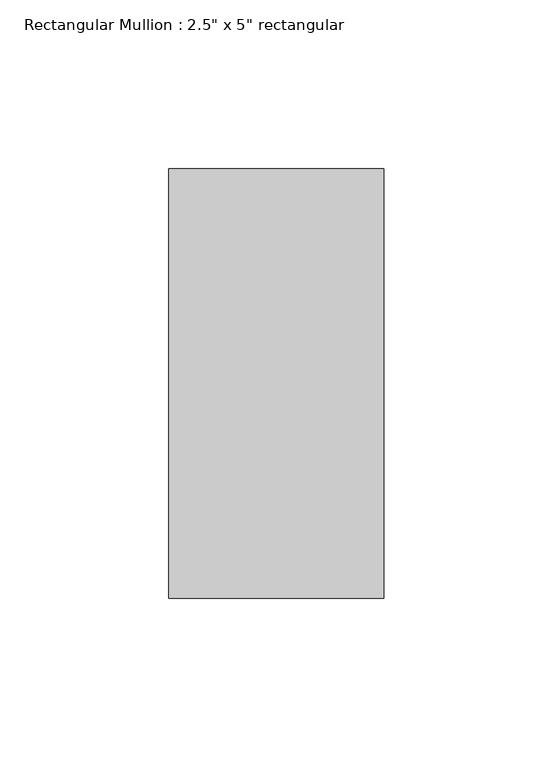
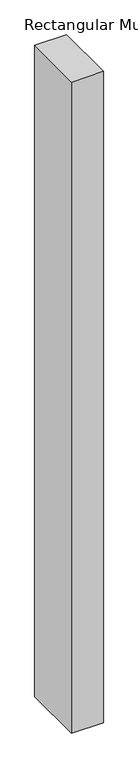
"""IFC4 building model written with IfcOpenShell, lengths in millimetres: member geometry."""

from ifc_helpers import new_model, si_unit, frame, origin, place, context, project, spatial, polyline, outline, extrude, source, transform, mapped, element, save


def member_554b6236(model_context):
    return source(origin(), model_context, "Body", "SweptSolid", [
        extrude(outline(polyline([(31.75, 63.5), (31.75, -63.5), (-31.75, -63.5), (-31.75, 63.5), (31.75, 63.5)])), frame((0.0, 0.0, -1371.6000002), z_axis=(0.0, 0.0, 1.0), x_axis=(1.0, 0.0, 0.0)), (0.0, 0.0, 1.0), 1371.6000002),
    ])


if __name__ == "__main__":
    model = new_model("IFC4")
    model_context = context("Model", 3, world=origin())
    ifc_project = project(units=[si_unit("LENGTHUNIT", "METRE", prefix="MILLI")], contexts=[model_context])
    site = spatial("IfcSite", under=ifc_project)
    building = spatial("IfcBuilding", under=site)
    placement = place(None, origin())
    member_shape = member_554b6236(model_context)
    element("IfcMember", 1, ObjectType="Rectangular Mullion : 2.5\" x 5\" rectangular", at=placement, inside=building, context=model_context, shape_type="MappedRepresentation", body=[
        mapped(member_shape, transform((0.0, 0.0, 0.0), x_axis=(1.0, 0.0, 0.0), y_axis=(0.0, 1.0, 0.0), z_axis=(0.0, 0.0, 1.0))),
    ])
    save(model, "model.ifc")

# Revit data of these elements
# Type "Rectangular Mullion : 2.5\" x 5\" rectangular"
#   built-in parameter 1007304 = 0.416667 (stored number, unit not read)
#   built-in parameter 1007301 = 0.104167 (stored number, unit not read)
#   built-in parameter 1007300 = 0.104167 (stored number, unit not read)
# Element 1 (IfcMember, "Rectangular Mullion : 2.5\" x 5\" rectangular")
#   Materials on its faces: "metal black"
# Materials
#   "metal black": class "Generic", colour RGB 120 120 120, transparency 0, Cost = 0
